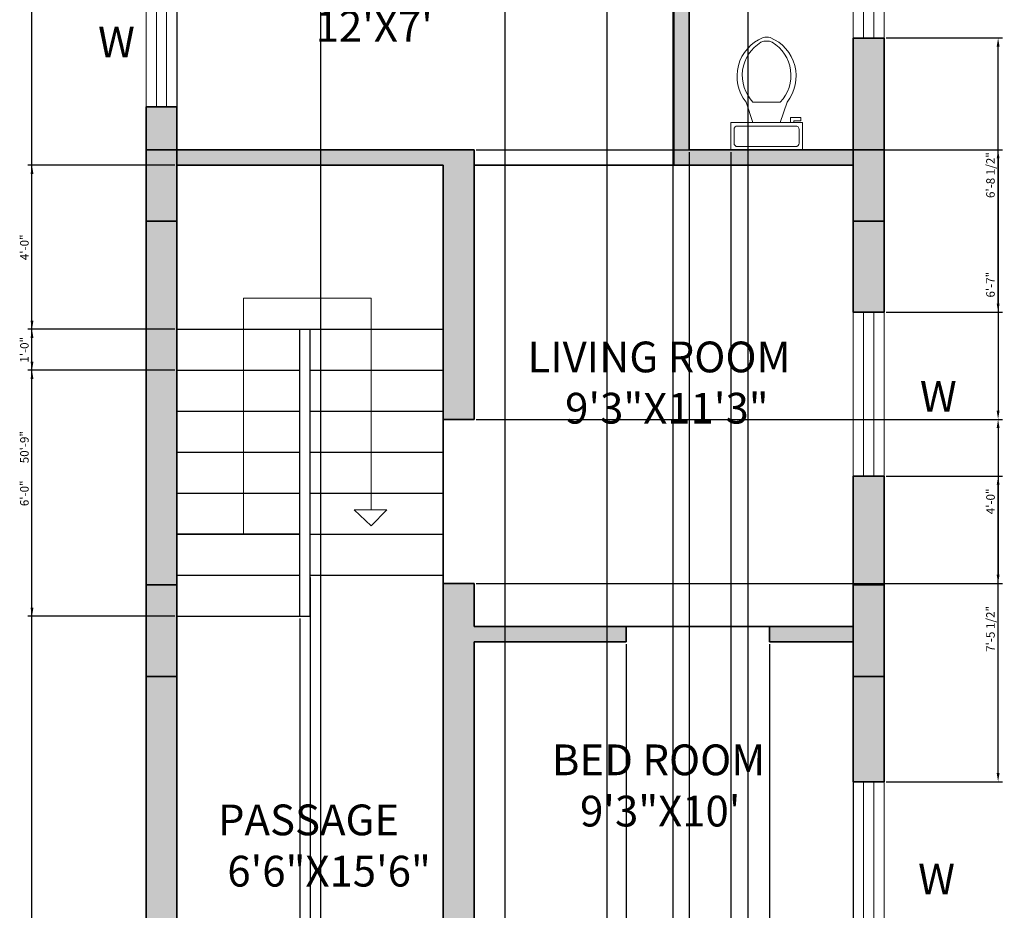
# Model space of a CAD drawing. Units: inches. Extents: x 4888 to 5178, y 5041 to 5743.
# Tile 2 of 3: x 4890 to 5178, y 5245 to 5506. Entities that reach past the tile are written whole.
import ezdxf

# ---------------------------------------------------------------- set-up
doc = ezdxf.new("R2010")
doc.units = ezdxf.units.IN
for name, color, linetype, lineweight in [('A-ANNO-DIMS', 2, 'Continuous', 18), ('A-ANNO-SYMB', 7, 'Continuous', 18), ('A-ANNO-TEXT', 7, 'Continuous', 18), ('A-AREA-IDEN', 7, 'Continuous', 18), ('A-COLS', 7, 'Continuous', 35), ('A-FLOR-FIXT', 9, 'Continuous', 18), ('A-FLOR-STRS', 7, 'Continuous', 25), ('A-WALL', 7, 'Continuous', 35), ('A-WALL-PATT', 8, 'Continuous', 13)]:
    doc.layers.add(name, color=color, linetype=linetype, lineweight=lineweight)
doc.layers.add('A-COLS-PATT', color=18, linetype='Continuous', lineweight=13, true_color=0x000000)
doc.layers.add('A-GLAZ', color=31, linetype='Continuous', lineweight=18, true_color=0xfecc66)
doc.styles.get("Standard").update_dxf_attribs({"font": 'arial.ttf'})
doc.dimstyles.new('ISO-25', dxfattribs={"dimtxt": 2.5, "dimasz": 2.5, "dimexe": 1.25, "dimexo": 0.625, "dimtad": 1, "dimlunit": 3, "dimtxsty": 'Standard', "dimcen": 2.5, "dimadec": 0, "dimazin": 0, "dimtfac": 1, "dimtmove": 0, "dimatfit": 3, "dimfxl": 1, "dimarcsym": 0})

# ---------------------------------------------------------------- blocks, each defined once
blk = doc.blocks.new('Toilet - top')
for p, q in [((9.5, -6), (9.5, -2)), ((-10, -8.5), (-8, -8.5)), ((-10, -9.5), (-10, -8.5)), ((-8, -8.5), (-8, -8)), ((-7, -8), (-7, -9.5)), ((-4, -8), (-6, -14)), ((4, -8), (6, -14)), ((-7, -9.5), (-10, -9.5)), ((4, -14), (-4, -14))]:
    blk.add_line(p, q)
blk.add_lwpolyline([(10.5, -8), (10.5, 0), (-10.5, 0), (-10.5, -8)], close=True)
for points in [[(-9.5, -2), (-9.5, -6)], [(8.5, -1), (-8.5, -1)], [(-8.5, -7), (8.5, -7)]]:
    blk.add_lwpolyline(points)
for centre, radius, start, end in [((-8.62, -1.88), 0.884, 81.8699, 188.1301), ((8.62, -1.88), 0.884, 351.8699, 98.1301), ((-8.62, -6.12), 0.884, 171.8699, 278.1301), ((8.62, -6.12), 0.884, 261.8699, 8.1301), ((3.52, -21.58), 12.17, 141.4691, 247.9714), ((4.2, -21.82), 11.33, 136.3677, 238.9468), ((-3.52, -21.58), 12.17, 292.0284, 38.5307), ((-4.2, -21.82), 11.33, 301.053, 43.6321), ((0, -27.88), 4, 245.7318, 294.2682), ((0, -29), 4, 254.8605, 285.1395)]:
    blk.add_arc(centre, radius, start, end)
blk = doc.blocks.new('WIN-48IN')
for p, q in [((0, 9), (0, 0)), ((48, 9), (0, 9)), ((48, 0), (48, 9)), ((48, 6), (0, 6)), ((48, 3), (0, 3)), ((0, 0), (48, 0))]:
    blk.add_line(p, q)
blk = doc.blocks.new('VENT-24IN')
for p, q in [((0, 24), (0, 0)), ((9, 24), (0, 24)), ((3, 0), (3, 24)), ((6, 0), (6, 24)), ((9, 0), (9, 24)), ((0, 0), (9, 0))]:
    blk.add_line(p, q)
blk = doc.blocks.new('*D17')
at = {"layer": 'A-ANNO-DIMS', "color": 0, "lineweight": -2, "transparency": 16777216}
for p, q in [((4926.22, 5685.01), (4892.19, 5685.01)), ((4893.44, 5078.51), (4893.44, 5682.51)), ((4926.22, 5076.01), (4892.19, 5076.01))]:
    blk.add_line(p, q, dxfattribs=at)
at = {"layer": 'A-ANNO-DIMS', "color": 0, "transparency": 16777216}
for points in [[(4893.03, 5682.51), (4893.86, 5682.51), (4893.44, 5685.01)], [(4893.03, 5078.51), (4893.86, 5078.51), (4893.44, 5076.01)]]:
    blk.add_solid(points, dxfattribs=at)
at = {"layer": 'Defpoints', "color": 0, "transparency": 16777216}
for p in [(4893.44, 5685.01), (4926.84, 5685.01), (4926.84, 5076.01)]:
    blk.add_point(p, dxfattribs=at)
at = {"layer": 'A-ANNO-DIMS', "color": 0, "transparency": 16777216, "insert": (4891.54, 5380.51), "char_height": 2.5, "attachment_point": 5, "rotation": 90}
blk.add_mtext('50\'-9"', dxfattribs=at)
blk = doc.blocks.new('*D24')
at = {"layer": 'A-ANNO-DIMS', "color": 0, "lineweight": -2, "transparency": 16777216}
for p, q in [((5143.47, 5372.01), (5177.49, 5372.01)), ((5176.24, 5285.11), (5176.24, 5369.51)), ((5143.47, 5282.61), (5177.49, 5282.61))]:
    blk.add_line(p, q, dxfattribs=at)
at = {"layer": 'A-ANNO-DIMS', "color": 0, "transparency": 16777216}
for points in [[(5175.83, 5369.51), (5176.66, 5369.51), (5176.24, 5372.01)], [(5175.83, 5285.11), (5176.66, 5285.11), (5176.24, 5282.61)]]:
    blk.add_solid(points, dxfattribs=at)
at = {"layer": 'Defpoints', "color": 0, "transparency": 16777216}
for p in [(5142.84, 5372.01), (5176.24, 5372.01), (5142.84, 5282.61)]:
    blk.add_point(p, dxfattribs=at)
at = {"layer": 'A-ANNO-DIMS', "color": 0, "transparency": 16777216, "insert": (5174.33, 5327.31), "char_height": 2.5, "attachment_point": 5, "rotation": 90}
blk.add_mtext('7\'-5 1/2"', dxfattribs=at)
blk = doc.blocks.new('*D25')
at = {"layer": 'A-ANNO-DIMS', "color": 0, "lineweight": -2, "transparency": 16777216}
for p, q in [((5143.47, 5500.27), (5177.49, 5500.27)), ((5176.24, 5422.51), (5176.24, 5497.77)), ((5143.47, 5420.01), (5177.49, 5420.01))]:
    blk.add_line(p, q, dxfattribs=at)
at = {"layer": 'A-ANNO-DIMS', "color": 0, "transparency": 16777216}
for points in [[(5175.83, 5497.77), (5176.66, 5497.77), (5176.24, 5500.27)], [(5175.83, 5422.51), (5176.66, 5422.51), (5176.24, 5420.01)]]:
    blk.add_solid(points, dxfattribs=at)
at = {"layer": 'Defpoints', "color": 0, "transparency": 16777216}
for p in [(5142.84, 5500.27), (5176.24, 5500.27), (5142.84, 5420.01)]:
    blk.add_point(p, dxfattribs=at)
at = {"layer": 'A-ANNO-DIMS', "color": 0, "transparency": 16777216, "insert": (5174.33, 5460.14), "char_height": 2.5, "attachment_point": 5, "rotation": 90}
blk.add_mtext('6\'-8 1/2"', dxfattribs=at)
blk = doc.blocks.new('*D26')
at = {"layer": 'A-ANNO-DIMS', "color": 0, "lineweight": -2, "transparency": 16777216}
for p, q in [((4935.22, 5463.01), (4892.19, 5463.01)), ((4893.44, 5417.51), (4893.44, 5460.51)), ((4935.22, 5415.01), (4892.19, 5415.01))]:
    blk.add_line(p, q, dxfattribs=at)
at = {"layer": 'A-ANNO-DIMS', "color": 0, "transparency": 16777216}
for points in [[(4893.03, 5460.51), (4893.86, 5460.51), (4893.44, 5463.01)], [(4893.03, 5417.51), (4893.86, 5417.51), (4893.44, 5415.01)]]:
    blk.add_solid(points, dxfattribs=at)
at = {"layer": 'Defpoints', "color": 0, "transparency": 16777216}
for p in [(4893.44, 5463.01), (4935.84, 5463.01), (4935.84, 5415.01)]:
    blk.add_point(p, dxfattribs=at)
at = {"layer": 'A-ANNO-DIMS', "color": 0, "transparency": 16777216, "insert": (4891.54, 5439.01), "char_height": 2.5, "attachment_point": 5, "rotation": 90}
blk.add_mtext('4\'-0"', dxfattribs=at)
blk = doc.blocks.new('*D27')
at = {"layer": 'A-ANNO-DIMS', "color": 0, "lineweight": -2, "transparency": 16777216}
for p, q in [((4935.22, 5415.01), (4892.19, 5415.01)), ((4893.44, 5405.51), (4893.44, 5412.51)), ((4935.22, 5403.01), (4892.19, 5403.01))]:
    blk.add_line(p, q, dxfattribs=at)
at = {"layer": 'A-ANNO-DIMS', "color": 0, "transparency": 16777216}
for points in [[(4893.03, 5412.51), (4893.86, 5412.51), (4893.44, 5415.01)], [(4893.03, 5405.51), (4893.86, 5405.51), (4893.44, 5403.01)]]:
    blk.add_solid(points, dxfattribs=at)
at = {"layer": 'Defpoints', "color": 0, "transparency": 16777216}
for p in [(4893.44, 5415.01), (4935.84, 5415.01), (4935.84, 5403.01)]:
    blk.add_point(p, dxfattribs=at)
at = {"layer": 'A-ANNO-DIMS', "color": 0, "transparency": 16777216, "insert": (4891.54, 5409.01), "char_height": 2.5, "attachment_point": 5, "rotation": 90}
blk.add_mtext('1\'-0"', dxfattribs=at)
blk = doc.blocks.new('*D28')
at = {"layer": 'A-ANNO-DIMS', "color": 0, "lineweight": -2, "transparency": 16777216}
for p, q in [((4935.84, 5330.38), (4935.84, 5041.36)), ((4971.84, 5330.38), (4971.84, 5041.36)), ((4938.34, 5042.61), (4969.34, 5042.61))]:
    blk.add_line(p, q, dxfattribs=at)
at = {"layer": 'A-ANNO-DIMS', "color": 0, "transparency": 16777216}
for points in [[(4938.34, 5043.02), (4938.34, 5042.19), (4935.84, 5042.61)], [(4969.34, 5043.02), (4969.34, 5042.19), (4971.84, 5042.61)]]:
    blk.add_solid(points, dxfattribs=at)
at = {"layer": 'Defpoints', "color": 0, "transparency": 16777216}
for p in [(4935.84, 5331.01), (4971.84, 5331.01), (4971.84, 5042.61)]:
    blk.add_point(p, dxfattribs=at)
at = {"layer": 'A-ANNO-DIMS', "color": 0, "transparency": 16777216, "insert": (4953.84, 5044.51), "char_height": 2.5, "attachment_point": 5}
blk.add_mtext('3\'-0"', dxfattribs=at)
blk = doc.blocks.new('*D29')
at = {"layer": 'A-ANNO-DIMS', "color": 0, "lineweight": -2, "transparency": 16777216}
for p, q in [((5067.37, 5322.88), (5067.37, 5041.36)), ((5109.37, 5322.88), (5109.37, 5041.36)), ((5069.87, 5042.61), (5106.87, 5042.61))]:
    blk.add_line(p, q, dxfattribs=at)
at = {"layer": 'A-ANNO-DIMS', "color": 0, "transparency": 16777216}
for points in [[(5069.87, 5043.02), (5069.87, 5042.19), (5067.37, 5042.61)], [(5106.87, 5043.02), (5106.87, 5042.19), (5109.37, 5042.61)]]:
    blk.add_solid(points, dxfattribs=at)
at = {"layer": 'Defpoints', "color": 0, "transparency": 16777216}
for p in [(5067.37, 5323.51), (5109.37, 5323.51), (5109.37, 5042.61)]:
    blk.add_point(p, dxfattribs=at)
at = {"layer": 'A-ANNO-DIMS', "color": 0, "transparency": 16777216, "insert": (5088.37, 5044.51), "char_height": 2.5, "attachment_point": 5}
blk.add_mtext('3\'-6"', dxfattribs=at)
blk = doc.blocks.new('*D30')
at = {"layer": 'A-ANNO-DIMS', "color": 0, "lineweight": -2, "transparency": 16777216}
for p, q in [((5109.37, 5322.88), (5109.37, 5041.36)), ((5133.84, 5322.88), (5133.84, 5041.36)), ((5131.34, 5042.61), (5111.87, 5042.61))]:
    blk.add_line(p, q, dxfattribs=at)
at = {"layer": 'A-ANNO-DIMS', "color": 0, "transparency": 16777216}
for points in [[(5111.87, 5043.02), (5111.87, 5042.19), (5109.37, 5042.61)], [(5131.34, 5043.02), (5131.34, 5042.19), (5133.84, 5042.61)]]:
    blk.add_solid(points, dxfattribs=at)
at = {"layer": 'Defpoints', "color": 0, "transparency": 16777216}
for p in [(5109.37, 5323.51), (5133.84, 5323.51), (5109.37, 5042.61)]:
    blk.add_point(p, dxfattribs=at)
at = {"layer": 'A-ANNO-DIMS', "color": 0, "transparency": 16777216, "insert": (5121.61, 5044.52), "char_height": 2.5, "attachment_point": 5}
blk.add_mtext('2\'-0 1/2"', dxfattribs=at)
blk = doc.blocks.new('*D31')
at = {"layer": 'A-ANNO-DIMS', "color": 0, "lineweight": -2, "transparency": 16777216}
for p, q in [((5023.47, 5388.65), (5177.49, 5388.65)), ((5176.24, 5386.15), (5176.24, 5343.15)), ((5023.47, 5340.65), (5177.49, 5340.65))]:
    blk.add_line(p, q, dxfattribs=at)
at = {"layer": 'A-ANNO-DIMS', "color": 0, "transparency": 16777216}
for points in [[(5175.83, 5386.15), (5176.66, 5386.15), (5176.24, 5388.65)], [(5175.83, 5343.15), (5176.66, 5343.15), (5176.24, 5340.65)]]:
    blk.add_solid(points, dxfattribs=at)
at = {"layer": 'Defpoints', "color": 0, "transparency": 16777216}
for p in [(5022.84, 5388.65), (5022.84, 5340.65), (5176.24, 5340.65)]:
    blk.add_point(p, dxfattribs=at)
at = {"layer": 'A-ANNO-DIMS', "color": 0, "transparency": 16777216, "insert": (5174.34, 5364.65), "char_height": 2.5, "attachment_point": 5, "rotation": 90}
blk.add_mtext('4\'-0"', dxfattribs=at)
blk = doc.blocks.new('*D32')
at = {"layer": 'A-ANNO-DIMS', "color": 0, "lineweight": -2, "transparency": 16777216}
for p, q in [((4977.89, 5550.88), (4977.89, 5041.36)), ((5031.84, 5550.88), (5031.84, 5041.36)), ((4980.39, 5042.61), (5029.34, 5042.61))]:
    blk.add_line(p, q, dxfattribs=at)
at = {"layer": 'A-ANNO-DIMS', "color": 0, "transparency": 16777216}
for points in [[(4980.39, 5043.02), (4980.39, 5042.19), (4977.89, 5042.61)], [(5029.34, 5043.02), (5029.34, 5042.19), (5031.84, 5042.61)]]:
    blk.add_solid(points, dxfattribs=at)
at = {"layer": 'Defpoints', "color": 0, "transparency": 16777216}
for p in [(4977.89, 5551.51), (5031.84, 5551.51), (5031.84, 5042.61)]:
    blk.add_point(p, dxfattribs=at)
at = {"layer": 'A-ANNO-DIMS', "color": 0, "transparency": 16777216, "insert": (5004.87, 5044.51), "char_height": 2.5, "attachment_point": 5}
blk.add_mtext('4\'-6"', dxfattribs=at)
blk = doc.blocks.new('*D36')
at = {"layer": 'A-ANNO-DIMS', "color": 0, "lineweight": -2, "transparency": 16777216}
for p, q in [((5081.08, 5204.13), (5081.08, 5719.66)), ((5083.58, 5718.41), (5100.61, 5718.41)), ((5103.11, 5204.13), (5103.11, 5719.66))]:
    blk.add_line(p, q, dxfattribs=at)
at = {"layer": 'A-ANNO-DIMS', "color": 0, "transparency": 16777216}
for points in [[(5083.58, 5718.82), (5083.58, 5717.99), (5081.08, 5718.41)], [(5100.61, 5718.82), (5100.61, 5717.99), (5103.11, 5718.41)]]:
    blk.add_solid(points, dxfattribs=at)
at = {"layer": 'Defpoints', "color": 0, "transparency": 16777216}
for p in [(5103.11, 5718.41), (5081.08, 5203.51), (5103.11, 5203.51)]:
    blk.add_point(p, dxfattribs=at)
at = {"layer": 'A-ANNO-DIMS', "color": 0, "transparency": 16777216, "insert": (5092.09, 5720.31), "char_height": 2.5, "attachment_point": 5}
blk.add_mtext('1\'-10"', dxfattribs=at)
blk = doc.blocks.new('*D39')
at = {"layer": 'A-ANNO-DIMS', "color": 0, "lineweight": -2, "transparency": 16777216}
for p, q in [((4935.84, 5555.38), (4935.84, 5041.36)), ((4977.89, 5555.38), (4977.89, 5041.36)), ((4938.34, 5042.61), (4975.39, 5042.61))]:
    blk.add_line(p, q, dxfattribs=at)
at = {"layer": 'A-ANNO-DIMS', "color": 0, "transparency": 16777216}
for points in [[(4938.34, 5043.02), (4938.34, 5042.19), (4935.84, 5042.61)], [(4975.39, 5043.02), (4975.39, 5042.19), (4977.89, 5042.61)]]:
    blk.add_solid(points, dxfattribs=at)
at = {"layer": 'Defpoints', "color": 0, "transparency": 16777216}
for p in [(4935.84, 5556.01), (4977.89, 5556.01), (4977.89, 5042.61)]:
    blk.add_point(p, dxfattribs=at)
at = {"layer": 'A-ANNO-DIMS', "color": 0, "transparency": 16777216, "insert": (4956.87, 5044.51), "char_height": 2.5, "attachment_point": 5}
blk.add_mtext('3\'-6"', dxfattribs=at)
blk = doc.blocks.new('*D40')
at = {"layer": 'A-ANNO-DIMS', "color": 0, "lineweight": -2, "transparency": 16777216}
for p, q in [((5061.84, 5204.13), (5061.84, 5719.66)), ((5064.34, 5718.41), (5078.58, 5718.41)), ((5081.08, 5204.13), (5081.08, 5719.66))]:
    blk.add_line(p, q, dxfattribs=at)
at = {"layer": 'A-ANNO-DIMS', "color": 0, "transparency": 16777216}
for points in [[(5064.34, 5718.82), (5064.34, 5717.99), (5061.84, 5718.41)], [(5078.58, 5718.82), (5078.58, 5717.99), (5081.08, 5718.41)]]:
    blk.add_solid(points, dxfattribs=at)
at = {"layer": 'Defpoints', "color": 0, "transparency": 16777216}
for p in [(5081.08, 5718.41), (5061.84, 5203.51), (5081.08, 5203.51)]:
    blk.add_point(p, dxfattribs=at)
at = {"layer": 'A-ANNO-DIMS', "color": 0, "transparency": 16777216, "insert": (5071.46, 5720.29), "char_height": 2.5, "attachment_point": 5}
blk.add_mtext('1\'-7"', dxfattribs=at)
blk = doc.blocks.new('*D50')
at = {"layer": 'A-ANNO-DIMS', "color": 0, "lineweight": -2, "transparency": 16777216}
for p, q in [((5085.84, 5466.88), (5085.84, 5041.36)), ((5097.97, 5466.88), (5097.97, 5041.36)), ((5095.47, 5042.61), (5088.34, 5042.61))]:
    blk.add_line(p, q, dxfattribs=at)
at = {"layer": 'A-ANNO-DIMS', "color": 0, "transparency": 16777216}
for points in [[(5088.34, 5043.02), (5088.34, 5042.19), (5085.84, 5042.61)], [(5095.47, 5043.02), (5095.47, 5042.19), (5097.97, 5042.61)]]:
    blk.add_solid(points, dxfattribs=at)
at = {"layer": 'Defpoints', "color": 0, "transparency": 16777216}
for p in [(5085.84, 5467.51), (5097.97, 5467.51), (5085.84, 5042.61)]:
    blk.add_point(p, dxfattribs=at)
at = {"layer": 'A-ANNO-DIMS', "color": 0, "transparency": 16777216, "insert": (5091.91, 5044.51), "char_height": 2.5, "attachment_point": 5}
blk.add_mtext('1\'-0"', dxfattribs=at)
blk = doc.blocks.new('*D51')
at = {"layer": 'A-ANNO-DIMS', "color": 0, "lineweight": -2, "transparency": 16777216}
for p, q in [((4971.84, 5330.38), (4971.84, 5041.36)), ((4974.84, 5330.38), (4974.84, 5041.36)), ((4969.34, 5042.61), (4966.84, 5042.61)), ((4971.84, 5042.61), (4974.84, 5042.61)), ((4977.34, 5042.61), (4987.74, 5042.61))]:
    blk.add_line(p, q, dxfattribs=at)
at = {"layer": 'A-ANNO-DIMS', "color": 0, "transparency": 16777216}
for points in [[(4969.34, 5043.02), (4969.34, 5042.19), (4971.84, 5042.61)], [(4977.34, 5043.02), (4977.34, 5042.19), (4974.84, 5042.61)]]:
    blk.add_solid(points, dxfattribs=at)
at = {"layer": 'Defpoints', "color": 0, "transparency": 16777216}
for p in [(4971.84, 5331.01), (4974.84, 5331.01), (4974.84, 5042.61)]:
    blk.add_point(p, dxfattribs=at)
at = {"layer": 'A-ANNO-DIMS', "color": 0, "transparency": 16777216, "insert": (4983.79, 5044.51), "char_height": 2.5, "attachment_point": 5}
blk.add_mtext('0\'-3"', dxfattribs=at)
blk = doc.blocks.new('*D52')
at = {"layer": 'A-ANNO-DIMS', "color": 0, "lineweight": -2, "transparency": 16777216}
for p, q in [((4974.84, 5342.38), (4974.84, 5041.36)), ((5013.84, 5342.38), (5013.84, 5041.36)), ((4977.34, 5042.61), (5011.34, 5042.61))]:
    blk.add_line(p, q, dxfattribs=at)
at = {"layer": 'A-ANNO-DIMS', "color": 0, "transparency": 16777216}
for points in [[(4977.34, 5043.02), (4977.34, 5042.19), (4974.84, 5042.61)], [(5011.34, 5043.02), (5011.34, 5042.19), (5013.84, 5042.61)]]:
    blk.add_solid(points, dxfattribs=at)
at = {"layer": 'Defpoints', "color": 0, "transparency": 16777216}
for p in [(4974.84, 5343.01), (5013.84, 5343.01), (5013.84, 5042.61)]:
    blk.add_point(p, dxfattribs=at)
at = {"layer": 'A-ANNO-DIMS', "color": 0, "transparency": 16777216, "insert": (4994.34, 5044.51), "char_height": 2.5, "attachment_point": 5}
blk.add_mtext('3\'-3"', dxfattribs=at)
blk = doc.blocks.new('*D53')
at = {"layer": 'A-ANNO-DIMS', "color": 0, "lineweight": -2, "transparency": 16777216}
for p, q in [((4935.22, 5403.01), (4892.19, 5403.01)), ((4893.44, 5333.51), (4893.44, 5400.51)), ((4935.22, 5331.01), (4892.19, 5331.01))]:
    blk.add_line(p, q, dxfattribs=at)
at = {"layer": 'A-ANNO-DIMS', "color": 0, "transparency": 16777216}
for points in [[(4893.03, 5400.51), (4893.86, 5400.51), (4893.44, 5403.01)], [(4893.03, 5333.51), (4893.86, 5333.51), (4893.44, 5331.01)]]:
    blk.add_solid(points, dxfattribs=at)
at = {"layer": 'Defpoints', "color": 0, "transparency": 16777216}
for p in [(4893.44, 5403.01), (4935.84, 5403.01), (4935.84, 5331.01)]:
    blk.add_point(p, dxfattribs=at)
at = {"layer": 'A-ANNO-DIMS', "color": 0, "transparency": 16777216, "insert": (4891.54, 5367.01), "char_height": 2.5, "attachment_point": 5, "rotation": 90}
blk.add_mtext('6\'-0"', dxfattribs=at)
blk = doc.blocks.new('*D54')
at = {"layer": 'A-ANNO-DIMS', "color": 0, "lineweight": -2, "transparency": 16777216}
for p, q in [((5023.47, 5467.51), (5177.49, 5467.51)), ((5176.24, 5465.01), (5176.24, 5391.15)), ((5023.47, 5388.65), (5177.49, 5388.65))]:
    blk.add_line(p, q, dxfattribs=at)
at = {"layer": 'A-ANNO-DIMS', "color": 0, "transparency": 16777216}
for points in [[(5175.83, 5465.01), (5176.66, 5465.01), (5176.24, 5467.51)], [(5175.83, 5391.15), (5176.66, 5391.15), (5176.24, 5388.65)]]:
    blk.add_solid(points, dxfattribs=at)
at = {"layer": 'Defpoints', "color": 0, "transparency": 16777216}
for p in [(5022.84, 5467.51), (5022.84, 5388.65), (5176.24, 5388.65)]:
    blk.add_point(p, dxfattribs=at)
at = {"layer": 'A-ANNO-DIMS', "color": 0, "transparency": 16777216, "insert": (5174.34, 5428.08), "char_height": 2.5, "attachment_point": 5, "rotation": 90}
blk.add_mtext('6\'-7"', dxfattribs=at)

msp = doc.modelspace()

# ---------------------------------------------------------------- hatches: boundary and pattern name
at = {"layer": 'A-COLS-PATT'}
h = msp.add_hatch(color=256, dxfattribs=at)
h.dxf.hatch_style = 1
h.paths.add_polyline_path([(4935.844, 5685.006), (4926.844, 5685.006), (4926.844, 5669.086), (4935.844, 5669.086)])
h.paths.add_polyline_path([(5142.844, 5685.006), (5133.844, 5685.006), (5133.844, 5669.086), (5142.844, 5669.086)])
h.paths.add_polyline_path([(4935.844, 5467.506), (4926.844, 5467.506), (4926.844, 5455.506), (4926.844, 5446.68), (4935.844, 5446.68)])
h.paths.add_polyline_path([(5142.844, 5467.506), (5133.844, 5467.506), (5133.844, 5446.68), (5142.844, 5446.68)])
h.paths.add_polyline_path([(4935.844, 5340.228), (4926.844, 5340.228), (4926.844, 5313.351), (4935.844, 5313.351)])
h.paths.add_polyline_path([(4935.844, 5095.626), (4926.844, 5095.626), (4926.844, 5076.006), (4935.844, 5076.006)])
h.paths.add_polyline_path([(5142.844, 5095.626), (5133.844, 5095.626), (5133.844, 5076.006), (5142.844, 5076.006)])
h = msp.add_hatch(color=256, dxfattribs=at)
h.dxf.hatch_style = 1
h.paths.add_polyline_path([(5142.844, 5340.228), (5133.844, 5340.228), (5133.844, 5328.006), (5133.844, 5313.351), (5142.844, 5313.351)])
at = {"layer": 'A-WALL-PATT'}
h = msp.add_hatch(color=256, dxfattribs=at)
h.dxf.hatch_style = 1
h.paths.add_polyline_path([(5050.684, 5685.006), (4935.844, 5685.006), (4935.844, 5676.006), (5031.844, 5676.006), (5031.844, 5551.506), (5039.344, 5551.506), (5039.344, 5556.006), (5036.344, 5556.006), (5036.344, 5676.006), (5050.684, 5676.006)])
h.paths.add_polyline_path([(4935.844, 5669.086), (4926.844, 5669.086), (4926.844, 5610.401), (4935.844, 5610.401)])
h.paths.add_polyline_path([(5133.844, 5685.006), (5098.684, 5685.006), (5098.684, 5676.006), (5133.844, 5676.006)])
h.paths.add_polyline_path([(5142.844, 5669.086), (5133.844, 5669.086), (5133.844, 5556.006), (5109.899, 5556.006), (5109.899, 5551.506), (5133.844, 5551.506), (5133.844, 5524.266), (5142.844, 5524.266)])
h.paths.add_polyline_path([(4977.891, 5556.006), (4935.844, 5556.006), (4935.844, 5562.401), (4926.844, 5562.401), (4926.844, 5528.1), (4935.844, 5528.1), (4935.844, 5551.506), (4977.891, 5551.506)])
h.paths.add_polyline_path([(4935.844, 5480.1), (4926.844, 5480.1), (4926.844, 5467.506), (4935.844, 5467.506)])
h.paths.add_polyline_path([(5022.844, 5467.506), (4935.844, 5467.506), (4935.844, 5463.006), (5013.844, 5463.006), (5013.844, 5388.655), (5022.844, 5388.655)])
h.paths.add_polyline_path([(5133.844, 5467.506), (5085.844, 5467.506), (5085.844, 5551.506), (5091.899, 5551.506), (5091.899, 5556.006), (5081.344, 5556.006), (5081.344, 5463.006), (5133.844, 5463.006)])
h.paths.add_polyline_path([(5142.844, 5500.266), (5133.844, 5500.266), (5133.844, 5467.506), (5142.844, 5467.506)])
h.paths.add_polyline_path([(5142.844, 5446.68), (5133.844, 5446.68), (5133.844, 5420.006), (5142.844, 5420.006)])
h.paths.add_polyline_path([(5022.844, 5323.506), (5067.366, 5323.506), (5067.366, 5328.006), (5022.844, 5328.006), (5022.844, 5340.655), (5013.844, 5340.655), (5013.844, 5137.506), (5061.844, 5137.506), (5061.844, 5122.915), (5070.844, 5122.915), (5070.844, 5137.506), (5133.844, 5137.506), (5133.844, 5119.626), (5142.844, 5119.626), (5142.844, 5158.641), (5133.844, 5158.641), (5133.844, 5146.506), (5070.844, 5146.506), (5070.844, 5194.506), (5081.079, 5194.506), (5081.079, 5203.506), (5061.844, 5203.506), (5061.844, 5146.506), (5022.844, 5146.506)])
h.paths.add_polyline_path([(4935.844, 5313.351), (4926.844, 5313.351), (4926.844, 5095.626), (4935.844, 5095.626)])
h.paths.add_polyline_path([(4935.844, 5446.68), (4926.844, 5446.68), (4926.844, 5340.228), (4935.844, 5340.228)])
h.paths.add_polyline_path([(5142.844, 5372.006), (5133.844, 5372.006), (5133.844, 5340.228), (5142.844, 5340.228)])
h.paths.add_polyline_path([(5133.844, 5328.006), (5109.366, 5328.006), (5109.366, 5323.506), (5133.844, 5323.506)], flags=17)
h.paths.add_polyline_path([(5142.844, 5313.351), (5133.844, 5313.351), (5133.844, 5282.61), (5142.844, 5282.61)], flags=17)
h.paths.add_polyline_path([(5142.844, 5234.61), (5133.844, 5234.61), (5133.844, 5203.506), (5103.109, 5203.506), (5103.109, 5194.506), (5133.844, 5194.506), (5133.844, 5182.641), (5142.844, 5182.641)], flags=17)
h.paths.add_polyline_path([(5133.844, 5085.006), (4935.844, 5085.006), (4935.844, 5076.006), (5133.844, 5076.006)])
h.paths.add_polyline_path([(5070.844, 5094.96), (5061.844, 5094.96), (5061.844, 5085.006), (5070.844, 5085.006)])

# ---------------------------------------------------------------- linework, layer by layer
at = {"layer": 'A-ANNO-SYMB'}
for p, q in [((4955.344, 5361.69), (4955.344, 5424.16)), ((4955.344, 5424.16), (4992.738, 5424.16)), ((4992.738, 5424.16), (4992.738, 5362.176)), ((4955.344, 5355.006), (4955.344, 5361.69)), ((4992.738, 5362.176), (4987.791, 5362.176)), ((4987.791, 5362.176), (4992.738, 5357.515)), ((4992.738, 5357.515), (4997.349, 5362.176)), ((4997.349, 5362.176), (4992.738, 5362.176)), ((4935.844, 5355.006), (4955.344, 5355.006))]:
    msp.add_line(p, q, dxfattribs=at)
at = {"layer": 'A-COLS'}
for p, q in [((4926.844, 5467.506), (4926.844, 5455.506)), ((4926.844, 5446.68), (4935.844, 5446.68)), ((5133.844, 5446.68), (5142.844, 5446.68)), ((4935.844, 5340.228), (4926.844, 5340.228)), ((5133.844, 5340.228), (5142.844, 5340.228)), ((4935.844, 5313.351), (4926.844, 5313.351)), ((5133.844, 5313.351), (5142.844, 5313.351))]:
    msp.add_line(p, q, dxfattribs=at)
at = {"layer": 'A-FLOR-STRS'}
for p, q in [((4935.844, 5415.006), (5013.844, 5415.006)), ((4971.844, 5331.006), (4971.844, 5415.006)), ((4974.844, 5331.006), (4974.844, 5415.006)), ((4935.844, 5403.006), (4971.844, 5403.006)), ((4974.844, 5403.006), (5013.844, 5403.006)), ((4935.844, 5391.006), (4971.844, 5391.006)), ((4974.844, 5391.006), (5013.844, 5391.006)), ((4935.844, 5379.006), (4971.844, 5379.006)), ((4974.844, 5379.006), (5013.844, 5379.006)), ((4935.844, 5367.006), (4971.844, 5367.006)), ((4974.844, 5367.006), (5013.844, 5367.006)), ((4935.844, 5355.006), (4971.844, 5355.006)), ((4971.844, 5355.006), (4935.844, 5355.006)), ((4974.844, 5355.006), (5013.844, 5355.006)), ((4935.844, 5343.006), (4971.844, 5343.006)), ((4974.844, 5343.006), (5013.844, 5343.006)), ((4935.844, 5331.006), (4974.844, 5331.006))]:
    msp.add_line(p, q, dxfattribs=at)
at = {"layer": 'A-WALL'}
for p, q in [((5081.344, 5556.006), (5081.344, 5463.006)), ((5085.844, 5551.506), (5085.844, 5467.506)), ((5133.844, 5500.266), (5142.844, 5500.266)), ((5133.844, 5500.266), (5133.844, 5467.506)), ((5142.844, 5500.266), (5142.844, 5420.006)), ((4926.844, 5076.006), (4926.844, 5480.1)), ((4926.844, 5480.1), (4935.844, 5480.1)), ((4926.844, 5455.506), (4926.844, 5480.1)), ((4935.844, 5467.506), (4935.844, 5480.1)), ((4926.844, 5467.506), (5022.844, 5467.506)), ((4935.844, 5076.006), (4935.844, 5467.506)), ((5022.844, 5467.506), (5022.844, 5388.655)), ((5085.844, 5467.506), (5142.844, 5467.506)), ((5133.844, 5467.506), (5133.844, 5420.006)), ((4935.844, 5463.006), (5013.844, 5463.006)), ((5013.844, 5463.006), (5013.844, 5137.506)), ((5022.844, 5463.006), (5133.844, 5463.006)), ((5133.844, 5420.006), (5142.844, 5420.006)), ((5013.844, 5388.655), (5022.844, 5388.655)), ((5133.844, 5372.006), (5142.844, 5372.006)), ((5133.844, 5372.006), (5133.844, 5328.006)), ((5142.844, 5372.006), (5142.844, 5282.61)), ((5013.844, 5340.655), (5022.844, 5340.655)), ((5022.844, 5340.655), (5022.844, 5328.006)), ((5022.844, 5328.006), (5133.844, 5328.006)), ((5067.366, 5328.006), (5067.366, 5323.506)), ((5109.366, 5328.006), (5109.366, 5323.506)), ((5133.844, 5328.006), (5133.844, 5282.61)), ((5022.844, 5323.506), (5067.366, 5323.506)), ((5022.844, 5323.506), (5022.844, 5146.506)), ((5109.366, 5323.506), (5133.844, 5323.506)), ((4935.844, 5300.256), (4935.844, 5269.506)), ((4935.844, 5300.256), (4935.844, 5300.256)), ((4935.844, 5300.256), (4935.844, 5269.506)), ((5133.844, 5282.61), (5142.844, 5282.61)), ((4935.844, 5269.506), (4935.844, 5278.053))]:
    msp.add_line(p, q, dxfattribs=at)

# ---------------------------------------------------------------- block references
at = {"layer": 'A-FLOR-FIXT', "rotation": 180}
msp.add_blockref('Toilet - top', (5108.471, 5467.506), dxfattribs=at)
at = {"layer": 'A-GLAZ'}
for p, rotation in [((4935.844, 5480.1), 89.9999999999992), ((5142.844, 5372.006), 90.00000000000249), ((5142.844, 5234.61), 90.00000000000003)]:
    msp.add_blockref('WIN-48IN', p, dxfattribs=dict(at, rotation=rotation))
msp.add_blockref('VENT-24IN', (5133.844, 5500.266), dxfattribs=at)

# ---------------------------------------------------------------- texts
at = {"layer": 'A-ANNO-TEXT', "char_height": 9, "attachment_point": 1}
for insert in [(4912.776, 5503.584), (5153.347, 5399.857), (5152.829, 5258.61)]:
    msp.add_mtext_dynamic_manual_height_columns('W', width=76.41803, gutter_width=12.5, heights=[0], dxfattribs=dict(at, insert=insert))
at = {"layer": 'A-AREA-IDEN', "char_height": 9, "attachment_point": 1}
for s, width, heights, insert in [(" DINING \\P  12'X7'", 113.95373, [67.058], (4970.97, 5523.183)), ('  LIVING ROOM\\P      9\'3"X11\'3"', 257.56561, [134.915], (5032.996, 5411.418)), (' BED ROOM\\P    9\'3"X10\'', 110.16218, [64.743], (5042.868, 5293.497)), ('PASSAGE\\P 6\'6"X15\'6"', 86.76309, [64.951], (4947.876, 5275.921))]:
    msp.add_mtext_dynamic_manual_height_columns(s, width=width, gutter_width=12.5, heights=heights, dxfattribs=dict(at, insert=insert))

# ---------------------------------------------------------------- dimensions: what is measured, and where the dimension line sits
at = {"layer": 'A-ANNO-DIMS'}
for base, p1, p2, picture, middle in [((5081.079, 5718.406), (5061.844, 5203.506), (5081.079, 5203.506), '*D40', (5071.462, 5720.286)), ((5103.109, 5718.406), (5081.079, 5203.506), (5103.109, 5203.506), '*D36', (5092.094, 5720.307)), ((4977.891, 5042.606), (4935.844, 5556.006), (4977.891, 5556.006), '*D39', (4956.867, 5044.508)), ((5031.844, 5042.606), (4977.891, 5551.506), (5031.844, 5551.506), '*D32', (5004.867, 5044.507)), ((5085.844, 5042.606), (5097.971, 5467.506), (5085.844, 5467.506), '*D50', (5091.907, 5044.507)), ((5013.844, 5042.606), (4974.844, 5343.006), (5013.844, 5343.006), '*D52', (4994.344, 5044.508)), ((4971.844, 5042.606), (4935.844, 5331.006), (4971.844, 5331.006), '*D28', (4953.844, 5044.508)), ((4974.844, 5042.606), (4971.844, 5331.006), (4974.844, 5331.006), '*D51', (4983.792, 5044.508)), ((5109.366, 5042.606), (5067.366, 5323.506), (5109.366, 5323.506), '*D29', (5088.366, 5044.508)), ((5109.366, 5042.606), (5133.844, 5323.506), (5109.366, 5323.506), '*D30', (5121.605, 5044.524))]:
    dim = msp.add_linear_dim(base=base, p1=p1, p2=p2, dimstyle='ISO-25', override={"dimdec": 1, "dimlfac": 1, "dimrnd": 0, "dimzin": 1, "dimdsep": 46, "dimlunit": 4, "dimfrac": 2}, dxfattribs=at)
    dim.commit()
    dim.dimension.update_dxf_attribs({"geometry": picture, "text_midpoint": middle})
for base, p1, p2, picture, middle in [((4893.444, 5685.006), (4926.844, 5076.006), (4926.844, 5685.006), '*D17', (4891.542, 5380.506)), ((5176.244, 5500.266), (5142.844, 5420.006), (5142.844, 5500.266), '*D25', (5174.326, 5460.136)), ((5176.244, 5388.655), (5022.844, 5467.506), (5022.844, 5388.655), '*D54', (5174.342, 5428.08)), ((4893.444, 5463.006), (4935.844, 5415.006), (4935.844, 5463.006), '*D26', (4891.542, 5439.006)), ((4893.444, 5415.006), (4935.844, 5403.006), (4935.844, 5415.006), '*D27', (4891.542, 5409.006)), ((4893.444, 5403.006), (4935.844, 5331.006), (4935.844, 5403.006), '*D53', (4891.542, 5367.006)), ((5176.244, 5340.655), (5022.844, 5388.655), (5022.844, 5340.655), '*D31', (5174.342, 5364.655)), ((5176.244, 5372.006), (5142.844, 5282.61), (5142.844, 5372.006), '*D24', (5174.326, 5327.308))]:
    dim = msp.add_linear_dim(base=base, p1=p1, p2=p2, angle=90, dimstyle='ISO-25', override={"dimdec": 1, "dimlfac": 1, "dimrnd": 0, "dimzin": 1, "dimdsep": 46, "dimlunit": 4, "dimfrac": 2}, dxfattribs=at)
    dim.commit()
    dim.dimension.update_dxf_attribs({"geometry": picture, "text_midpoint": middle})

doc.saveas('drawing.dxf')
